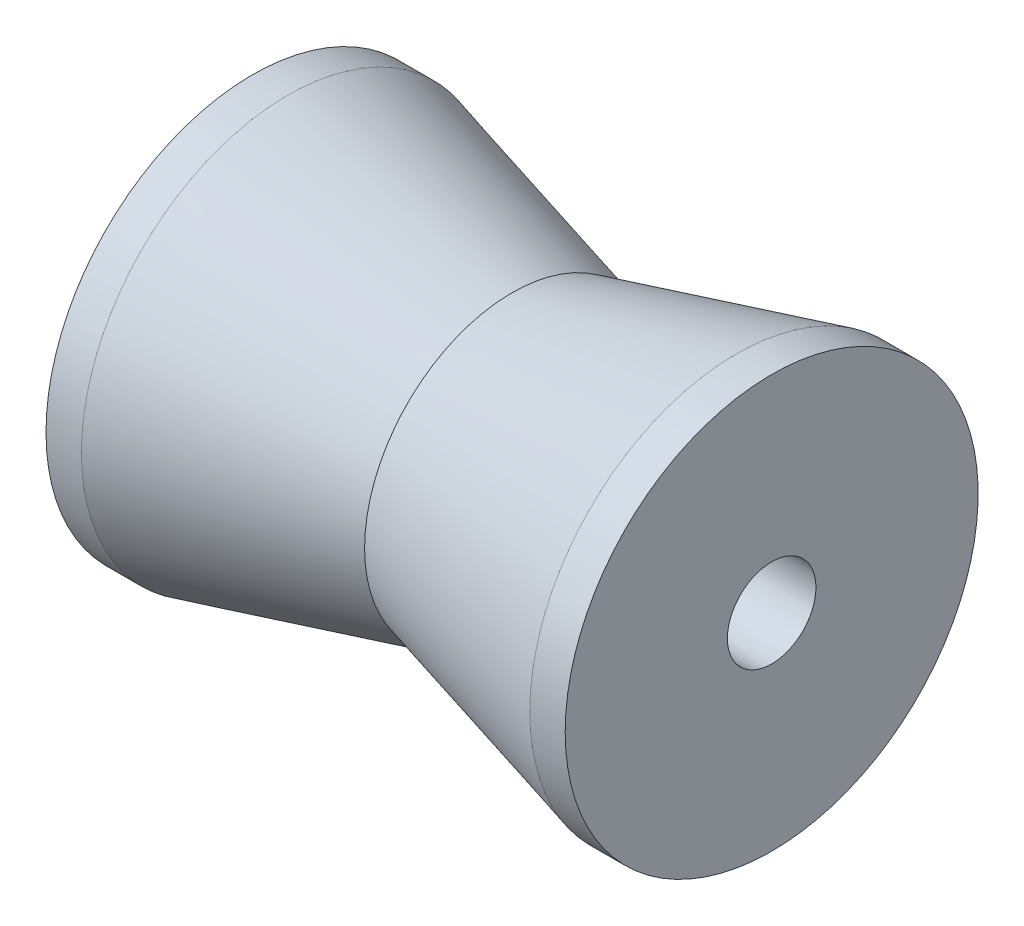
from build123d import *


with BuildPart() as part:
    # Roller Profile Sketch → Roller Body Revolve (revolve)
    with BuildSketch(Plane.XY, mode=Mode.PRIVATE) as roller_body_revolve_sk:
        Polygon((0, 50), (-38, 60), (-44, 60), (-44, 32.5), (44, 32.5), (44, 60), (38, 60), align=None)
    revolve(roller_body_revolve_sk.sketch.rotate(Axis((-44, 25, 0), (1, 0, 0)), 90), axis=Axis((-44, 25, 0), (1, 0, 0)))


solid = part.part
